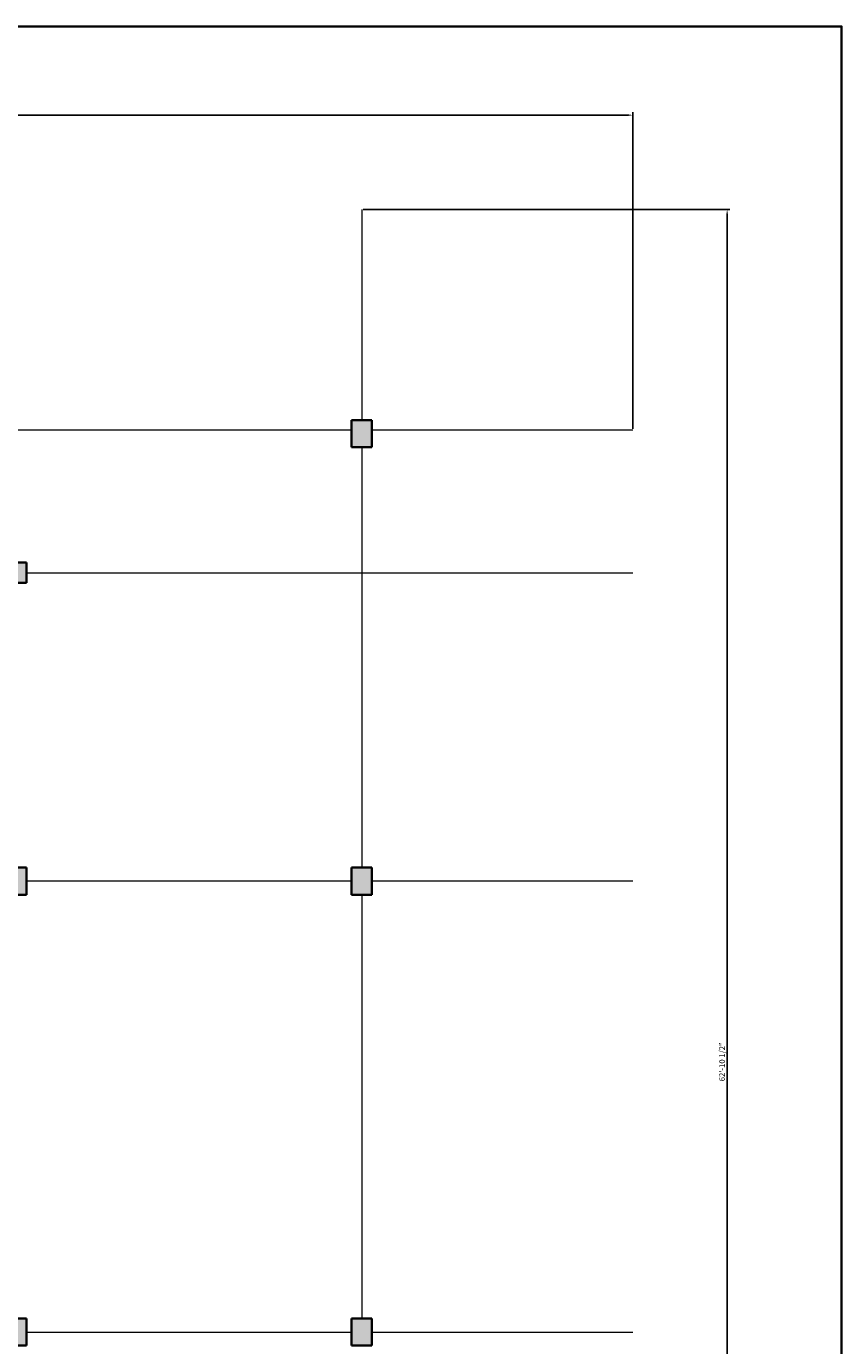
# Model space of a CAD drawing. Units: inches. Extents: x 6038 to 7543, y 3772 to 5131.
# Tile 14 of 14: x 7182 to 7543, y 4547 to 5131. Entities that reach past the tile are written whole.
import ezdxf

# ---------------------------------------------------------------- set-up
doc = ezdxf.new("R2010")
doc.units = ezdxf.units.IN
for name, color, linetype, lineweight in [('A-ANNO-DIMS', 4, 'Continuous', 18), ('A-ANNO-TTLB', 1, 'Continuous', 35), ('S-COLS', 7, 'Continuous', 35), ('S-COLS-PATT', 9, 'Continuous', 13), ('S-GRID', 6, 'Continuous', 13)]:
    doc.layers.add(name, color=color, linetype=linetype, lineweight=lineweight)
doc.styles.get("Standard").update_dxf_attribs({"font": 'arial.ttf'})
doc.dimstyles.new('ISO-25', dxfattribs={"dimtxt": 2.5, "dimasz": 2.5, "dimexe": 1.25, "dimexo": 0.625, "dimtad": 1, "dimdec": 0, "dimlunit": 3, "dimtxsty": 'Standard', "dimcen": 2.5, "dimadec": 0, "dimazin": 0, "dimtfac": 1, "dimtdec": 0, "dimtmove": 0, "dimatfit": 3, "dimfxl": 1, "dimarcsym": 0})

# ---------------------------------------------------------------- blocks, each defined once
blk = doc.blocks.new('COL-9X9')
for p, q in [((0, 9), (9, 9)), ((0, 0), (0, 9)), ((9, 9), (9, 0)), ((9, 0), (0, 0))]:
    blk.add_line(p, q)
blk = doc.blocks.new('COL-9X12')
for p, q in [((0, 12), (9, 12)), ((0, 0), (0, 12)), ((9, 12), (9, 0)), ((9, 0), (0, 0))]:
    blk.add_line(p, q)
blk = doc.blocks.new('*D92')
at = {"layer": 'A-ANNO-DIMS', "color": 0, "lineweight": -2, "transparency": 16777216}
for p, q in [((6853.8, 4952.74), (6853.8, 5092.84)), ((6856.3, 5091.59), (7447.59, 5091.59)), ((7450.09, 4952.74), (7450.09, 5092.84))]:
    blk.add_line(p, q, dxfattribs=at)
at = {"layer": 'A-ANNO-DIMS', "color": 0, "transparency": 16777216}
for points in [[(6856.3, 5092), (6856.3, 5091.17), (6853.8, 5091.59)], [(7447.59, 5092), (7447.59, 5091.17), (7450.09, 5091.59)]]:
    blk.add_solid(points, dxfattribs=at)
at = {"layer": 'Defpoints', "color": 0, "transparency": 16777216}
for p in [(7450.09, 5091.59), (6853.8, 4952.12), (7450.09, 4952.12)]:
    blk.add_point(p, dxfattribs=at)
at = {"layer": 'A-ANNO-DIMS', "color": 0, "transparency": 16777216, "insert": (7151.95, 5093.5), "char_height": 2.5, "attachment_point": 5}
blk.add_mtext('49\'-8 1/2"', dxfattribs=at)
blk = doc.blocks.new('*D93')
at = {"layer": 'A-ANNO-DIMS', "color": 0, "lineweight": -2, "transparency": 16777216}
for p, q in [((7330.71, 5049.84), (7493.09, 5049.84)), ((7491.84, 4298.03), (7491.84, 5047.34)), ((7330.71, 4295.53), (7493.09, 4295.53))]:
    blk.add_line(p, q, dxfattribs=at)
at = {"layer": 'A-ANNO-DIMS', "color": 0, "transparency": 16777216}
for points in [[(7491.43, 5047.34), (7492.26, 5047.34), (7491.84, 5049.84)], [(7491.43, 4298.03), (7492.26, 4298.03), (7491.84, 4295.53)]]:
    blk.add_solid(points, dxfattribs=at)
at = {"layer": 'Defpoints', "color": 0, "transparency": 16777216}
for p in [(7330.09, 5049.84), (7491.84, 5049.84), (7330.09, 4295.53)]:
    blk.add_point(p, dxfattribs=at)
at = {"layer": 'A-ANNO-DIMS', "color": 0, "transparency": 16777216, "insert": (7489.92, 4672.68), "char_height": 2.5, "attachment_point": 5, "rotation": 90}
blk.add_mtext('62\'-10 1/2"', dxfattribs=at)

msp = doc.modelspace()

# ---------------------------------------------------------------- hatches: boundary and pattern name
at = {"layer": 'S-COLS-PATT'}
h = msp.add_hatch(color=256, dxfattribs=at)
h.dxf.hatch_style = 1
h.paths.add_polyline_path([(7325.59, 4944.62), (7334.59, 4944.62), (7334.59, 4956.62), (7325.59, 4956.62)])
h.paths.add_polyline_path([(7334.59, 4746.62), (7334.59, 4758.62), (7325.59, 4758.62), (7325.59, 4746.62)])
h.paths.add_polyline_path([(7181.59, 4758.62), (7172.59, 4758.62), (7172.59, 4746.62), (7181.59, 4746.62)])
h.paths.add_polyline_path([(6983.59, 4758.62), (6974.59, 4758.62), (6974.59, 4746.62), (6983.59, 4746.62)])
h.paths.add_polyline_path([(6983.59, 4559.12), (6974.59, 4559.12), (6974.59, 4547.12), (6983.59, 4547.12)])
h.paths.add_polyline_path([(7181.59, 4559.12), (7172.59, 4559.12), (7172.59, 4547.12), (7181.59, 4547.12)])
h.paths.add_polyline_path([(7334.59, 4559.12), (7325.59, 4559.12), (7325.59, 4547.12), (7334.59, 4547.12)])
h = msp.add_hatch(color=256, dxfattribs=at)
h.dxf.hatch_style = 1
h.paths.add_polyline_path([(6974.59, 4884.62), (6983.59, 4884.62), (6983.59, 4893.62), (6974.59, 4893.62)])
h.paths.add_polyline_path([(7181.59, 4893.62), (7172.59, 4893.62), (7172.59, 4884.62), (7181.59, 4884.62)])
h.paths.add_polyline_path([(6983.59, 4436.12), (6983.59, 4445.12), (6974.59, 4445.12), (6974.59, 4436.12)])
h.paths.add_polyline_path([(7181.59, 4446.62), (7172.59, 4446.62), (7172.59, 4437.62), (7181.59, 4437.62)])
h.paths.add_polyline_path([(7325.59, 4436.12), (7334.59, 4436.12), (7334.59, 4445.12), (7325.59, 4445.12)])
h.paths.add_polyline_path([(7334.59, 4371.62), (7325.59, 4371.62), (7325.59, 4362.62), (7334.59, 4362.62)])
h.paths.add_polyline_path([(7181.59, 4362.62), (7181.59, 4371.62), (7172.59, 4371.62), (7172.59, 4362.62)])
h.paths.add_polyline_path([(6974.59, 4362.62), (6983.59, 4362.62), (6983.59, 4371.62), (6974.59, 4371.62)])

# ---------------------------------------------------------------- linework, layer by layer
at = {"layer": 'A-ANNO-TTLB'}
msp.add_lwpolyline([(6037.83, 5130.86), (7542.53, 5130.86), (7542.53, 3772.09), (6037.83, 3772.09)], close=True, dxfattribs=at)
at = {"layer": 'S-GRID'}
for p, q in [((7330.09, 5049.84), (7330.09, 4956.62)), ((7325.59, 4952.12), (6853.8, 4952.12)), ((7450.09, 4952.12), (7334.59, 4952.12)), ((7330.09, 4944.62), (7330.09, 4758.62)), ((7181.59, 4889.12), (7450.09, 4889.12)), ((7325.59, 4752.62), (7181.59, 4752.62)), ((7450.09, 4752.62), (7334.59, 4752.62)), ((7330.09, 4746.62), (7330.09, 4559.12)), ((7181.59, 4553.12), (7325.59, 4553.12)), ((7334.59, 4553.12), (7450.09, 4553.12))]:
    msp.add_line(p, q, dxfattribs=at)

# ---------------------------------------------------------------- block references
at = {"layer": 'S-COLS'}
for name, p in [('COL-9X12', (7325.59, 4944.62)), ('COL-9X9', (7172.59, 4884.62)), ('COL-9X12', (7172.59, 4746.62)), ('COL-9X12', (7325.59, 4746.62)), ('COL-9X12', (7172.59, 4547.12)), ('COL-9X12', (7325.59, 4547.12))]:
    msp.add_blockref(name, p, dxfattribs=at)

# ---------------------------------------------------------------- dimensions: what is measured, and where the dimension line sits
at = {"layer": 'A-ANNO-DIMS'}
dim = msp.add_linear_dim(base=(7450.09, 5091.59), p1=(6853.8, 4952.12), p2=(7450.09, 4952.12), dimstyle='ISO-25', override={"dimdec": 1, "dimlfac": 1, "dimrnd": 0, "dimzin": 1, "dimdsep": 46, "dimlunit": 4, "dimfrac": 2}, dxfattribs=at)
dim.commit()
dim.dimension.update_dxf_attribs({"geometry": '*D92', "text_midpoint": (7151.95, 5093.5)})
dim = msp.add_linear_dim(base=(7491.84, 5049.84), p1=(7330.09, 4295.53), p2=(7330.09, 5049.84), angle=90, dimstyle='ISO-25', override={"dimdec": 1, "dimlfac": 1, "dimrnd": 0, "dimzin": 1, "dimdsep": 46, "dimlunit": 4, "dimfrac": 2}, dxfattribs=at)
dim.commit()
dim.dimension.update_dxf_attribs({"geometry": '*D93', "text_midpoint": (7489.92, 4672.68)})

doc.saveas('drawing.dxf')
